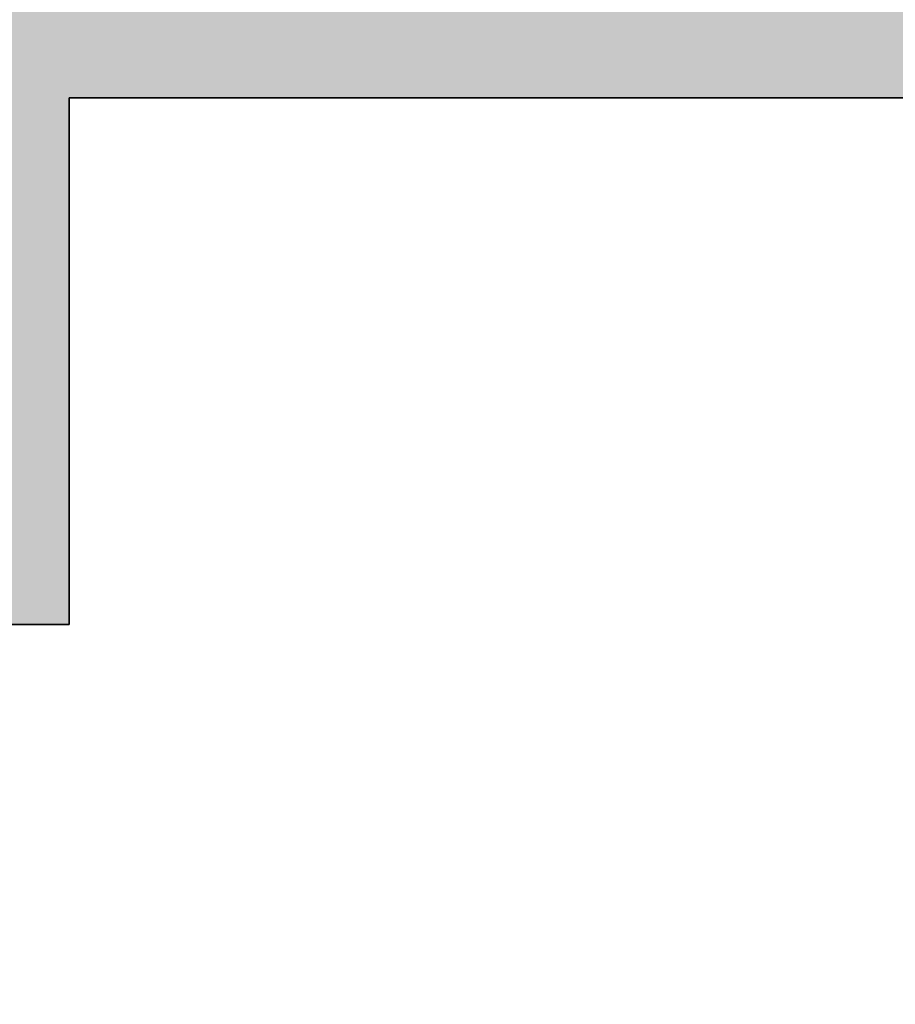
# Model space of a CAD drawing. Units: inches. Extents: x 638 to 1303, y 1 to 699.
# Tile 13 of 21: x 924 to 964, y 503 to 548. Entities that reach past the tile are written whole.
import ezdxf

# ---------------------------------------------------------------- set-up
doc = ezdxf.new("R2010")
doc.units = ezdxf.units.IN
doc.header["$MEASUREMENT"] = 0
doc.layers.add('A-ANNO-DIMS', color=2, linetype='Continuous', lineweight=18)
doc.layers.add('A-WALL', color=7, linetype='Continuous', lineweight=35)
doc.layers.add('A-WALL-PATT', color=143, linetype='Continuous', lineweight=13, true_color=0x7aafdf)
doc.styles.get("Standard").update_dxf_attribs({"font": 'arial.ttf'})
doc.dimstyles.get("Standard").update_dxf_attribs({"dimtxt": 8, "dimasz": 0.18, "dimexe": 0.18, "dimexo": 0.0625, "dimgap": 0.09, "dimtad": 0, "dimtih": 1, "dimtoh": 1, "dimdec": 4, "dimzin": 0, "dimdsep": 46, "dimlunit": 3, "dimtxsty": 'Standard', "dimcen": 0.09, "dimadec": 0, "dimazin": 0, "dimtfac": 1, "dimtdec": 4, "dimtofl": 0, "dimtmove": 0, "dimatfit": 3, "dimfxl": 1, "dimtolj": 1, "dimtzin": 0, "dimarcsym": 0})

# ---------------------------------------------------------------- blocks, each defined once
blk = doc.blocks.new('*D68')
at = {"layer": 'A-ANNO-DIMS', "color": 0, "lineweight": -2, "transparency": 16777216}
for p, q in [((908.943, 524.881), (908.943, 560.499)), ((909.123, 560.319), (922.058, 560.319)), ((922.238, 524.881), (922.238, 560.499)), ((922.238, 560.319), (922.418, 560.319))]:
    blk.add_line(p, q, dxfattribs=at)
at = {"layer": 'A-ANNO-DIMS', "color": 0, "transparency": 16777216}
for points in [[(909.123, 560.349), (909.123, 560.289), (908.943, 560.319)], [(922.058, 560.349), (922.058, 560.289), (922.238, 560.319)]]:
    blk.add_solid(points, dxfattribs=at)
at = {"layer": 'Defpoints', "color": 0, "transparency": 16777216}
for p in [(922.238, 560.319), (908.943, 524.819), (922.238, 524.819)]:
    blk.add_point(p, dxfattribs=at)
at = {"layer": 'A-ANNO-DIMS', "color": 0, "transparency": 16777216, "insert": (942.085, 560.319), "char_height": 8, "attachment_point": 5}
blk.add_mtext('\\A1;1\'-1 1/2"', dxfattribs=at)

msp = doc.modelspace()

# ---------------------------------------------------------------- hatches: boundary and pattern name
at = {"layer": 'A-WALL-PATT'}
h = msp.add_hatch(color=256, dxfattribs=at)
h.dxf.hatch_style = 1
h.paths.add_polyline_path([(973.34524, 629.81895), (793.35541, 629.81895), (793.35541, 620.81895), (850.23798, 620.81895), (922.23798, 620.81895), (922.23798, 524.81895), (908.94335, 524.81895), (908.94335, 520.31895), (926.73798, 520.31895), (926.73798, 544.31895), (979.3571, 544.31895), (979.3571, 548.81895), (926.73798, 548.81895), (926.73798, 620.81895), (973.34524, 620.81895)])
h.paths.add_polyline_path([(758.35541, 629.81895), (697.23798, 629.81895), (697.23798, 586.77451), (706.23798, 586.77451), (706.23798, 620.81895), (758.35541, 620.81895)])
h.paths.add_polyline_path([(1075.85281, 629.81895), (1003.34524, 629.81895), (1003.34524, 620.81895), (1046.73798, 620.81895), (1046.73798, 560.81895), (1046.73798, 548.81895), (1026.3571, 548.81895), (1026.3571, 544.31895), (1046.73798, 544.31895), (1046.73798, 486.87457), (1051.23798, 486.87457), (1051.23798, 556.31895), (1162.89753, 556.31895), (1162.89753, 560.81895), (1051.23798, 560.81895), (1051.23798, 620.81895), (1075.85281, 620.81895)])
h.paths.add_polyline_path([(1228.23798, 629.81895), (1105.85281, 629.81895), (1105.85281, 620.81895), (1219.23798, 620.81895), (1219.23798, 560.81895), (1197.89753, 560.81895), (1197.89753, 556.31895), (1219.23798, 556.31895), (1219.23798, 498.80084), (1228.23798, 498.80084)])
h.paths.add_polyline_path([(1051.23798, 439.87457), (1046.73798, 439.87457), (1046.73798, 407.81895), (1219.23798, 407.81895), (1219.23798, 381.66175), (1228.23798, 381.66175), (1228.23798, 451.80084), (1219.23798, 451.80084), (1219.23798, 412.31895), (1051.23798, 412.31895)])
h.paths.add_polyline_path([(1228.23798, 346.66175), (1219.23798, 346.66175), (1219.23798, 335.81895), (1046.73798, 335.81895), (1046.73798, 273.56895), (1051.23798, 273.56895), (1051.23798, 331.31895), (1219.23798, 331.31895), (1219.23798, 308.99654), (1228.23798, 308.99654)])
h.paths.add_polyline_path([(1228.23798, 261.99654), (1219.23798, 261.99654), (1219.23798, 211.31895), (1051.23798, 211.31895), (1051.23798, 226.56895), (1046.73798, 226.56895), (1046.73798, 211.31895), (983.84714, 211.31895), (983.84714, 206.81895), (1219.23798, 206.81895), (1219.23798, 166.83987), (1228.23798, 166.83987)])
h.paths.add_polyline_path([(1228.23798, 119.83987), (1219.23798, 119.83987), (1219.23798, 50.81895), (1197.89277, 50.81895), (1197.89277, 41.81895), (1228.23798, 41.81895)])
h.paths.add_polyline_path([(1162.89277, 50.81895), (1069.02949, 50.81895), (1069.02949, 41.81895), (1162.89277, 41.81895)])
h.paths.add_polyline_path([(1010.02949, 50.81895), (941.89631, 50.81895), (917.77455, 50.81895), (917.77455, 41.81895), (941.89631, 41.81895), (1010.02949, 41.81895)])
h.paths.add_polyline_path([(882.77455, 50.81895), (854.73798, 50.81895), (854.73798, 145.50379), (850.23798, 145.50379), (850.23798, 50.81895), (793.49755, 50.81895), (793.49755, 41.81895), (882.77455, 41.81895)])
h.paths.add_polyline_path([(746.49755, 50.81895), (706.23798, 50.81895), (706.23798, 96.57416), (697.23798, 96.57416), (697.23798, 41.81895), (746.49755, 41.81895)])
h.paths.add_polyline_path([(706.23798, 206.81895), (714.01165, 206.81895), (714.01165, 211.31895), (706.23798, 211.31895), (706.23798, 251.21966), (697.23798, 251.21966), (697.23798, 143.57416), (706.23798, 143.57416)])
h.paths.add_polyline_path([(923.84714, 211.31895), (854.73798, 211.31895), (854.73798, 397.8313), (850.23798, 397.8313), (850.23798, 388.31895), (747.9539, 388.31895), (747.9539, 383.81895), (850.23798, 383.81895), (850.23798, 311.81895), (706.23798, 311.81895), (706.23798, 342.78787), (697.23798, 342.78787), (697.23798, 281.21966), (706.23798, 281.21966), (706.23798, 307.31895), (850.23798, 307.31895), (850.23798, 211.31895), (749.01165, 211.31895), (749.01165, 206.81895), (850.23798, 206.81895), (850.23798, 192.50379), (854.73798, 192.50379), (854.73798, 206.81895), (923.84714, 206.81895)])
h.paths.add_polyline_path([(706.23798, 434.70471), (697.23798, 434.70471), (697.23798, 372.78787), (706.23798, 372.78787), (706.23798, 383.81895), (712.9539, 383.81895), (712.9539, 388.31895), (706.23798, 388.31895)])
h.paths.add_polyline_path([(706.23798, 520.31895), (850.23798, 520.31895), (850.23798, 444.8313), (854.73798, 444.8313), (854.73798, 520.31895), (861.94335, 520.31895), (861.94335, 524.81895), (706.23798, 524.81895), (706.23798, 551.77451), (697.23798, 551.77451), (697.23798, 481.70471), (706.23798, 481.70471)])

# ---------------------------------------------------------------- linework, layer by layer
at = {"layer": 'A-WALL'}
for p, q in [((926.73798, 520.31895), (926.73798, 544.31895)), ((979.3571, 544.31895), (926.73798, 544.31895)), ((926.73798, 520.31895), (908.94335, 520.31895))]:
    msp.add_line(p, q, dxfattribs=at)

# ---------------------------------------------------------------- dimensions: what is measured, and where the dimension line sits
at = {"layer": 'A-ANNO-DIMS'}
dim = msp.add_linear_dim(base=(922.23798, 560.31895), p1=(908.94335, 524.81895), p2=(922.23798, 524.81895), angle=0, dimstyle='Standard', override={"dimdec": 1, "dimlfac": 1, "dimrnd": 0, "dimzin": 1, "dimdsep": 46, "dimlunit": 4, "dimfrac": 2}, dxfattribs=at)
dim.commit()
dim.dimension.update_dxf_attribs({"geometry": '*D68', "text_midpoint": (942.08506, 560.31895)})

doc.saveas('drawing.dxf')
